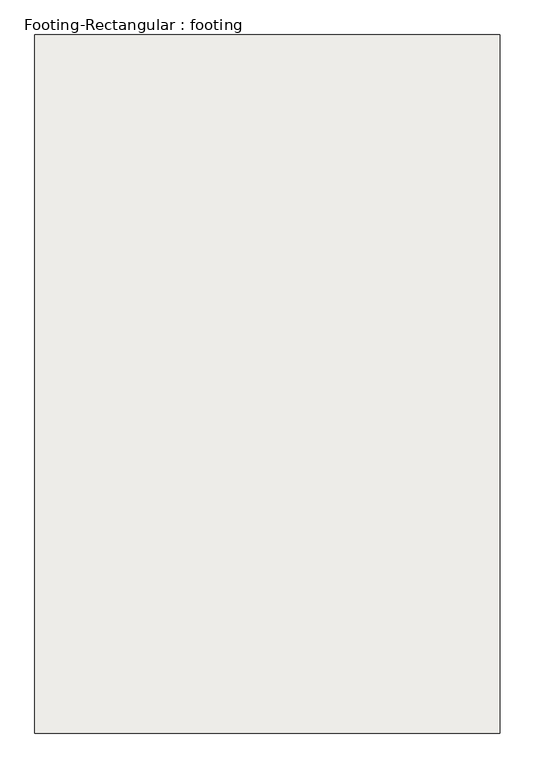
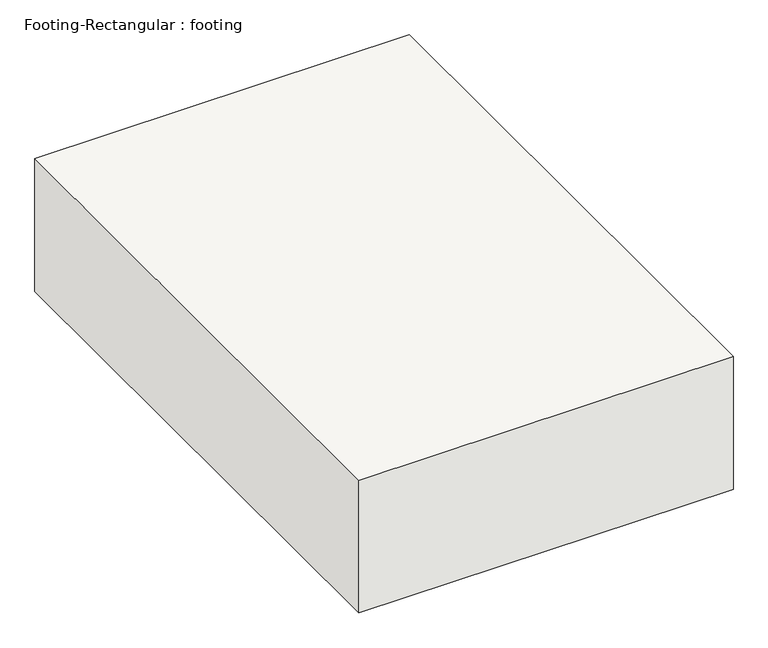
"""IFC4 building model written with IfcOpenShell, lengths in millimetres: slab geometry, Footing-Rectangular : footing."""

from ifc_helpers import new_model, si_unit, frame, origin, place, context, project, spatial, polyline, outline, extrude, source, transform, mapped, element, save


def footing_rectangular_footing_5ba74754(model_context):
    return source(origin(), model_context, "Body", "SweptSolid", [
        extrude(outline(polyline([(609.6, 914.4), (609.6, -914.4), (-609.6, -914.4), (-609.6, 914.4), (609.6, 914.4)])), frame((0.0, 0.0, -457.2), z_axis=(0.0, 0.0, 1.0), x_axis=(1.0, 0.0, 0.0)), (0.0, 0.0, 1.0), 457.2),
    ])


if __name__ == "__main__":
    model = new_model("IFC4")
    model_context = context("Model", 3, world=origin())
    ifc_project = project(units=[si_unit("LENGTHUNIT", "METRE", prefix="MILLI")], contexts=[model_context])
    site = spatial("IfcSite", under=ifc_project)
    building = spatial("IfcBuilding", under=site)
    placement = place(None, origin())
    footing_rectangular_footing_shape = footing_rectangular_footing_5ba74754(model_context)
    element("IfcSlab", 1, ObjectType="Footing-Rectangular : footing", at=placement, inside=building, context=model_context, shape_type="MappedRepresentation", body=[
        mapped(footing_rectangular_footing_shape, transform((0.0, 0.0, 0.0), x_axis=(1.0, 0.0, 0.0), y_axis=(0.0, 1.0, 0.0), z_axis=(0.0, 0.0, 1.0))),
    ])
    save(model, "model.ifc")

# Revit data of these elements
# Type "Footing-Rectangular : footing"
#   Assembly Code = "A1010100"
#   Width = 1219.2 mm
#   Length = 1828.8 mm
#   Foundation Thickness = 457.2 mm
#   Structural Material [instance default] = Concrete, Cast-in-Place gray
# Element 1 (IfcSlab, "Footing-Rectangular : footing")
#   Materials on its faces: "Concrete, Cast-in-Place gray"
# Materials
#   "Concrete, Cast-in-Place gray": class "Concrete", colour RGB 192 192 192, transparency 0, Description = "Cast-in-place concrete", Cost = 0
